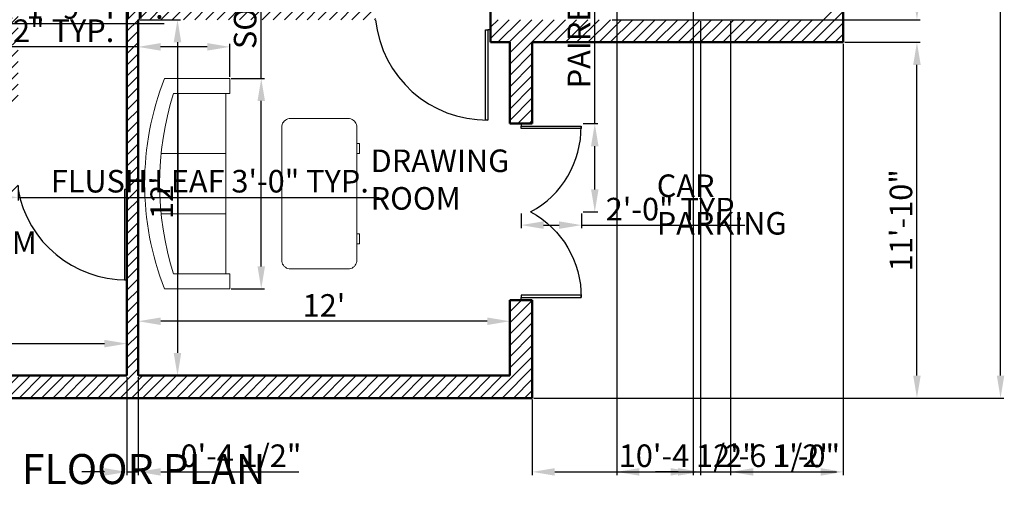
# Model space of a CAD drawing. Units: inches. Extents: x 5928 to 6612, y 5674 to 6320.
# Tile 2 of 5: x 6219 to 6612, y 5674 to 5862. Entities that reach past the tile are written whole.
import ezdxf

# ---------------------------------------------------------------- set-up
doc = ezdxf.new("R2010")
doc.units = ezdxf.units.IN
for name, color, linetype, lineweight in [('A-ANNO-DIMS', 2, 'Continuous', 18), ('A-ANNO-TEXT', 7, 'Continuous', 25), ('A-AREA-IDEN', 7, 'Continuous', 25), ('A-DOOR', 3, 'Continuous', 25), ('A-FURN', 8, 'Continuous', 18), ('A-WALL', 7, 'Continuous', 50), ('A-WALL-PATT', 252, 'Continuous', 13)]:
    doc.layers.add(name, color=color, linetype=linetype, lineweight=lineweight)
doc.styles.get("Standard").update_dxf_attribs({"font": 'arial.ttf'})
doc.dimstyles.new('ISO-25', dxfattribs={"dimtxt": 9, "dimasz": 9, "dimexe": 1.25, "dimexo": 0.625, "dimtad": 1, "dimdec": 1, "dimrnd": 9, "dimlunit": 3, "dimtxsty": 'Standard', "dimcen": 2.5, "dimadec": 0, "dimazin": 0, "dimtfac": 1, "dimtdec": 1, "dimtmove": 0, "dimatfit": 3, "dimfxl": 1, "dimarcsym": 0})

# ---------------------------------------------------------------- blocks, each defined once
blk = doc.blocks.new('Sofa - Roundback 7 ft.')
for p, q in [((-12.00002, -32.4421), (-12.00003, -6.5971)), ((11.99997, -32.4421), (11.99998, -6.5971)), ((-36.000027, -34), (-36.000027, -11.4696)), ((35.99998, -34), (35.99998, -11.4696)), ((-35.999844, -13.3819), (35.9998, -13.3819)), ((-36.000027, -32.4421), (35.99998, -32.4421))]:
    blk.add_line(p, q)
for points in [[(-36.000027, -34), (-42.000027, -34), (-42.000027, -8)], [(41.99998, -8), (41.99998, -34), (35.99998, -34)]]:
    blk.add_lwpolyline(points)
for centre, radius, start, end in [((0, -114.25), 114.25, 68.43141, 111.5686), ((-0.00001, -127.1968), 121.1968, 72.72033, 107.2797)]:
    blk.add_arc(centre, radius, start, end)
blk = doc.blocks.new('Desk - 30 x 60 in.')
for p, q in [((-26.999995, 0), (26.999995, 0)), ((-29.999995, -27), (-29.999995, -3)), ((29.999995, -3), (29.999995, -27)), ((26.999995, -30), (-26.999995, -30)), ((-20.000005, -30), (-20.000005, -31)), ((-20.000005, -31), (-16.000005, -31)), ((-16.000005, -31), (-16.000005, -30)), ((15.999995, -31), (15.999995, -30)), ((19.999995, -31), (15.999995, -31)), ((19.999995, -30), (19.999995, -31))]:
    blk.add_line(p, q)
for centre, start, end in [((-26.499995, -3.5), 98.1301, 171.8699), ((26.499995, -3.5), 8.130102, 81.8699), ((-26.499995, -26.5), 188.1301, 261.8699), ((26.499995, -26.5), 278.1301, 351.8699)]:
    blk.add_arc(centre, 3.535534, start, end)
blk = doc.blocks.new('*D20')
at = {"layer": 'A-ANNO-DIMS', "color": 0, "lineweight": -2, "transparency": 16777216}
for p, q in [((6117.76, 5720.89), (6117.76, 5734.25)), ((6261.76, 5720.89), (6261.76, 5734.25)), ((6126.76, 5733), (6252.76, 5733))]:
    blk.add_line(p, q, dxfattribs=at)
at = {"layer": 'A-ANNO-DIMS', "color": 0, "transparency": 16777216}
for points in [[(6126.76, 5734.5), (6126.76, 5731.5), (6117.76, 5733)], [(6252.76, 5734.5), (6252.76, 5731.5), (6261.76, 5733)]]:
    blk.add_solid(points, dxfattribs=at)
at = {"layer": 'Defpoints', "color": 0, "transparency": 16777216}
for p in [(6261.76, 5733), (6117.76, 5720.26), (6261.76, 5720.26)]:
    blk.add_point(p, dxfattribs=at)
at = {"layer": 'A-ANNO-DIMS', "color": 0, "transparency": 16777216, "insert": (6189.76, 5738.14), "char_height": 9, "attachment_point": 5}
blk.add_mtext("12'", dxfattribs=at)
blk = doc.blocks.new('*D21')
at = {"layer": 'A-ANNO-DIMS', "color": 0, "lineweight": -2, "transparency": 16777216}
for p, q in [((6266.88, 5862.26), (6283.21, 5862.26)), ((6281.96, 5853.26), (6281.96, 5729.26)), ((6266.88, 5720.26), (6283.21, 5720.26))]:
    blk.add_line(p, q, dxfattribs=at)
at = {"layer": 'A-ANNO-DIMS', "color": 0, "transparency": 16777216}
for points in [[(6280.46, 5853.26), (6283.46, 5853.26), (6281.96, 5862.26)], [(6280.46, 5729.26), (6283.46, 5729.26), (6281.96, 5720.26)]]:
    blk.add_solid(points, dxfattribs=at)
at = {"layer": 'Defpoints', "color": 0, "transparency": 16777216}
for p in [(6266.26, 5862.26), (6266.26, 5720.26), (6281.96, 5720.26)]:
    blk.add_point(p, dxfattribs=at)
at = {"layer": 'A-ANNO-DIMS', "color": 0, "transparency": 16777216, "insert": (6276.82, 5791.26), "char_height": 9, "attachment_point": 5, "rotation": 90}
blk.add_mtext("12'", dxfattribs=at)
blk = doc.blocks.new('*D22')
at = {"layer": 'A-ANNO-DIMS', "color": 0, "lineweight": -2, "transparency": 16777216}
for p, q in [((6266.26, 5720.89), (6266.26, 5743.18)), ((6405.76, 5741.93), (6275.26, 5741.93)), ((6414.76, 5720.89), (6414.76, 5743.18))]:
    blk.add_line(p, q, dxfattribs=at)
at = {"layer": 'A-ANNO-DIMS', "color": 0, "transparency": 16777216}
for points in [[(6275.26, 5743.43), (6275.26, 5740.43), (6266.26, 5741.93)], [(6405.76, 5743.43), (6405.76, 5740.43), (6414.76, 5741.93)]]:
    blk.add_solid(points, dxfattribs=at)
at = {"layer": 'Defpoints', "color": 0, "transparency": 16777216}
for p in [(6266.26, 5741.93), (6266.26, 5720.26), (6414.76, 5720.26)]:
    blk.add_point(p, dxfattribs=at)
at = {"layer": 'A-ANNO-DIMS', "color": 0, "transparency": 16777216, "insert": (6340.51, 5747.07), "char_height": 9, "attachment_point": 5}
blk.add_mtext("12'", dxfattribs=at)
blk = doc.blocks.new('*D37')
at = {"layer": 'A-ANNO-DIMS', "color": 0, "lineweight": -2, "transparency": 16777216}
for p, q in [((6497.65, 6228.26), (6612.14, 6228.26)), ((6610.89, 5720.26), (6610.89, 6219.26)), ((6424.38, 5711.26), (6612.14, 5711.26))]:
    blk.add_line(p, q, dxfattribs=at)
at = {"layer": 'A-ANNO-DIMS', "color": 0, "transparency": 16777216}
for points in [[(6609.39, 6219.26), (6612.39, 6219.26), (6610.89, 6228.26)], [(6609.39, 5720.26), (6612.39, 5720.26), (6610.89, 5711.26)]]:
    blk.add_solid(points, dxfattribs=at)
at = {"layer": 'Defpoints', "color": 0, "transparency": 16777216}
for p in [(6497.03, 6228.26), (6610.89, 6228.26), (6423.76, 5711.26)]:
    blk.add_point(p, dxfattribs=at)
at = {"layer": 'A-ANNO-DIMS', "color": 0, "transparency": 16777216, "insert": (6605.67, 5969.76), "char_height": 9, "attachment_point": 5, "rotation": 90}
blk.add_mtext('42\'-9"', dxfattribs=at)
blk = doc.blocks.new('DOOR-LEAF-36IN')
for p, q in [((0, 0), (0, 36)), ((0, 36), (1, 36)), ((1, 36), (1, 0)), ((-1, 0), (0, 0)), ((1, 0), (0, 0))]:
    blk.add_line(p, q)
blk = doc.blocks.new('DOOR-LEAF-FLUSH-36IN')
for p, q in [((0, 0), (-1, 0)), ((-1, 0), (-1, -36)), ((-1, -36), (0, -36))]:
    blk.add_line(p, q)
blk = doc.blocks.new('DOOR-PAIRED-LEAF-24IN')
for p, q in [((0, 0), (0, -1)), ((0, -1), (24, -1)), ((0, -2), (0, -1)), ((24, -2), (0, -2)), ((24, -1), (24, -2))]:
    blk.add_line(p, q)
blk.add_arc((-14.28, -1.5), 38.28, 298.2595, 0.7484)
blk = doc.blocks.new('*D49')
at = {"layer": 'A-ANNO-DIMS', "color": 0, "lineweight": -2, "transparency": 16777216}
for p, q in [((6191.35, 5865.09), (6191.35, 5859.51)), ((6212.35, 5865.09), (6212.35, 5859.51)), ((6200.35, 5860.76), (6203.35, 5860.76)), ((6212.35, 5860.76), (6276.61, 5860.76))]:
    blk.add_line(p, q, dxfattribs=at)
at = {"layer": 'A-ANNO-DIMS', "color": 0, "transparency": 16777216}
for points in [[(6200.35, 5862.26), (6200.35, 5859.26), (6191.35, 5860.76)], [(6203.35, 5862.26), (6203.35, 5859.26), (6212.35, 5860.76)]]:
    blk.add_solid(points, dxfattribs=at)
at = {"layer": 'Defpoints', "color": 0, "transparency": 16777216}
for p in [(6191.35, 5865.72), (6212.35, 5865.72), (6212.35, 5860.76)]:
    blk.add_point(p, dxfattribs=at)
at = {"layer": 'A-ANNO-DIMS', "color": 0, "transparency": 16777216, "insert": (6248.98, 5865.98), "char_height": 9, "attachment_point": 5}
blk.add_mtext('1\'-9" TYP.', dxfattribs=at)
blk = doc.blocks.new('*D54')
at = {"layer": 'A-ANNO-DIMS', "color": 0, "lineweight": -2, "transparency": 16777216}
for p, q in [((6315.43, 5838.83), (6315.43, 5941.63)), ((6303.46, 5838.83), (6316.68, 5838.83)), ((6315.43, 5763.83), (6315.43, 5829.83)), ((6303.46, 5754.83), (6316.68, 5754.83))]:
    blk.add_line(p, q, dxfattribs=at)
at = {"layer": 'A-ANNO-DIMS', "color": 0, "transparency": 16777216}
for points in [[(6313.93, 5829.83), (6316.93, 5829.83), (6315.43, 5838.83)], [(6313.93, 5763.83), (6316.93, 5763.83), (6315.43, 5754.83)]]:
    blk.add_solid(points, dxfattribs=at)
at = {"layer": 'Defpoints', "color": 0, "transparency": 16777216}
for p in [(6302.83, 5838.83), (6315.43, 5838.83), (6302.83, 5754.83)]:
    blk.add_point(p, dxfattribs=at)
at = {"layer": 'A-ANNO-DIMS', "color": 0, "transparency": 16777216, "insert": (6310.15, 5894.73), "char_height": 9, "attachment_point": 5, "rotation": 90}
blk.add_mtext('SOFA 7\'-0" TYP.', dxfattribs=at)
blk = doc.blocks.new('*D55')
at = {"layer": 'A-ANNO-DIMS', "color": 0, "lineweight": -2, "transparency": 16777216}
for p, q in [((6266.17, 5851.43), (6180.09, 5851.43)), ((6266.17, 5839.46), (6266.17, 5852.68)), ((6293.83, 5851.43), (6275.17, 5851.43)), ((6302.83, 5839.46), (6302.83, 5852.68))]:
    blk.add_line(p, q, dxfattribs=at)
at = {"layer": 'A-ANNO-DIMS', "color": 0, "transparency": 16777216}
for points in [[(6275.17, 5852.93), (6275.17, 5849.93), (6266.17, 5851.43)], [(6293.83, 5852.93), (6293.83, 5849.93), (6302.83, 5851.43)]]:
    blk.add_solid(points, dxfattribs=at)
at = {"layer": 'Defpoints', "color": 0, "transparency": 16777216}
for p in [(6266.17, 5851.43), (6266.17, 5838.83), (6302.83, 5838.83)]:
    blk.add_point(p, dxfattribs=at)
at = {"layer": 'A-ANNO-DIMS', "color": 0, "transparency": 16777216, "insert": (6218.63, 5856.72), "char_height": 9, "attachment_point": 5, "rotation": 360}
blk.add_mtext('3\'-0 1/2" TYP.', dxfattribs=at)
blk = doc.blocks.new('*D60')
at = {"layer": 'A-ANNO-DIMS', "color": 0, "lineweight": -2, "transparency": 16777216}
for p, q in [((6182.26, 5796.14), (6182.26, 5790.11)), ((6218.26, 5796.14), (6218.26, 5790.11)), ((6191.26, 5791.36), (6209.26, 5791.36)), ((6218.26, 5791.36), (6362.51, 5791.36))]:
    blk.add_line(p, q, dxfattribs=at)
at = {"layer": 'A-ANNO-DIMS', "color": 0, "transparency": 16777216}
for points in [[(6191.26, 5792.86), (6191.26, 5789.86), (6182.26, 5791.36)], [(6209.26, 5792.86), (6209.26, 5789.86), (6218.26, 5791.36)]]:
    blk.add_solid(points, dxfattribs=at)
at = {"layer": 'Defpoints', "color": 0, "transparency": 16777216}
for p in [(6182.26, 5796.76), (6218.26, 5796.76), (6218.26, 5791.36)]:
    blk.add_point(p, dxfattribs=at)
at = {"layer": 'A-ANNO-DIMS', "color": 0, "transparency": 16777216, "insert": (6294.88, 5796.65), "char_height": 9, "attachment_point": 5}
blk.add_mtext('FLUSH LEAF 3\'-0" TYP.', dxfattribs=at)
blk = doc.blocks.new('*D62')
at = {"layer": 'A-ANNO-DIMS', "color": 0, "lineweight": -2, "transparency": 16777216}
for p, q in [((6448.73, 5820.79), (6448.73, 5977.68)), ((6444.07, 5820.79), (6449.98, 5820.79)), ((6448.73, 5794.57), (6448.73, 5811.79)), ((6444.07, 5785.57), (6449.98, 5785.57))]:
    blk.add_line(p, q, dxfattribs=at)
at = {"layer": 'A-ANNO-DIMS', "color": 0, "transparency": 16777216}
for points in [[(6447.23, 5811.79), (6450.23, 5811.79), (6448.73, 5820.79)], [(6447.23, 5794.57), (6450.23, 5794.57), (6448.73, 5785.57)]]:
    blk.add_solid(points, dxfattribs=at)
at = {"layer": 'Defpoints', "color": 0, "transparency": 16777216}
for p in [(6443.45, 5820.79), (6448.73, 5820.79), (6443.45, 5785.57)]:
    blk.add_point(p, dxfattribs=at)
at = {"layer": 'A-ANNO-DIMS', "color": 0, "transparency": 16777216, "insert": (6443.58, 5903.73), "char_height": 9, "attachment_point": 5, "rotation": 90}
blk.add_mtext('PAIRED LEAF 2\'-11" TYP.', dxfattribs=at)
blk = doc.blocks.new('*D63')
at = {"layer": 'A-ANNO-DIMS', "color": 0, "lineweight": -2, "transparency": 16777216}
for p, q in [((6419.26, 5784.94), (6419.26, 5779.04)), ((6443.45, 5784.94), (6443.45, 5779.04)), ((6428.26, 5780.29), (6434.45, 5780.29)), ((6443.45, 5780.29), (6508.71, 5780.29))]:
    blk.add_line(p, q, dxfattribs=at)
at = {"layer": 'A-ANNO-DIMS', "color": 0, "transparency": 16777216}
for points in [[(6428.26, 5781.79), (6428.26, 5778.79), (6419.26, 5780.29)], [(6434.45, 5781.79), (6434.45, 5778.79), (6443.45, 5780.29)]]:
    blk.add_solid(points, dxfattribs=at)
at = {"layer": 'Defpoints', "color": 0, "transparency": 16777216}
for p in [(6419.26, 5785.57), (6443.45, 5785.57), (6443.45, 5780.29)]:
    blk.add_point(p, dxfattribs=at)
at = {"layer": 'A-ANNO-DIMS', "color": 0, "transparency": 16777216, "insert": (6480.58, 5785.51), "char_height": 9, "attachment_point": 5}
blk.add_mtext('2\'-0" TYP.', dxfattribs=at)
blk = doc.blocks.new('*D70')
at = {"layer": 'A-ANNO-DIMS', "color": 0, "lineweight": -2, "transparency": 16777216}
for p, q in [((6548.03, 5852.64), (6548.03, 5680.56)), ((6423.76, 5710.64), (6423.76, 5680.56)), ((6432.76, 5681.81), (6539.03, 5681.81))]:
    blk.add_line(p, q, dxfattribs=at)
at = {"layer": 'A-ANNO-DIMS', "color": 0, "transparency": 16777216}
for points in [[(6432.76, 5683.31), (6432.76, 5680.31), (6423.76, 5681.81)], [(6539.03, 5683.31), (6539.03, 5680.31), (6548.03, 5681.81)]]:
    blk.add_solid(points, dxfattribs=at)
at = {"layer": 'Defpoints', "color": 0, "transparency": 16777216}
for p in [(6548.03, 5853.26), (6423.76, 5711.26), (6548.03, 5681.81)]:
    blk.add_point(p, dxfattribs=at)
at = {"layer": 'A-ANNO-DIMS', "color": 0, "transparency": 16777216, "insert": (6485.89, 5687.09), "char_height": 9, "attachment_point": 5}
blk.add_mtext('10\'-4 1/2"', dxfattribs=at)
blk = doc.blocks.new('*D71')
at = {"layer": 'A-ANNO-DIMS', "color": 0, "lineweight": -2, "transparency": 16777216}
for p, q in [((6548.65, 5853.26), (6578.73, 5853.26)), ((6577.48, 5720.26), (6577.48, 5844.26)), ((6424.38, 5711.26), (6578.73, 5711.26))]:
    blk.add_line(p, q, dxfattribs=at)
at = {"layer": 'A-ANNO-DIMS', "color": 0, "transparency": 16777216}
for points in [[(6575.98, 5844.26), (6578.98, 5844.26), (6577.48, 5853.26)], [(6575.98, 5720.26), (6578.98, 5720.26), (6577.48, 5711.26)]]:
    blk.add_solid(points, dxfattribs=at)
at = {"layer": 'Defpoints', "color": 0, "transparency": 16777216}
for p in [(6548.03, 5853.26), (6577.48, 5853.26), (6423.76, 5711.26)]:
    blk.add_point(p, dxfattribs=at)
at = {"layer": 'A-ANNO-DIMS', "color": 0, "transparency": 16777216, "insert": (6572.26, 5782.26), "char_height": 9, "attachment_point": 5, "rotation": 90}
blk.add_mtext('11\'-10"', dxfattribs=at)
blk = doc.blocks.new('*D76')
at = {"layer": 'A-ANNO-DIMS', "color": 0, "lineweight": -2, "transparency": 16777216}
for p, q in [((6261.76, 5719.64), (6261.76, 5680.56)), ((6266.26, 5719.64), (6266.26, 5680.56)), ((6252.76, 5681.81), (6243.76, 5681.81)), ((6261.76, 5681.81), (6266.26, 5681.81)), ((6275.26, 5681.81), (6330.41, 5681.81))]:
    blk.add_line(p, q, dxfattribs=at)
at = {"layer": 'A-ANNO-DIMS', "color": 0, "transparency": 16777216}
for points in [[(6252.76, 5683.31), (6252.76, 5680.31), (6261.76, 5681.81)], [(6275.26, 5683.31), (6275.26, 5680.31), (6266.26, 5681.81)]]:
    blk.add_solid(points, dxfattribs=at)
at = {"layer": 'Defpoints', "color": 0, "transparency": 16777216}
for p in [(6261.76, 5720.26), (6266.26, 5720.26), (6266.26, 5681.81)]:
    blk.add_point(p, dxfattribs=at)
at = {"layer": 'A-ANNO-DIMS', "color": 0, "transparency": 16777216, "insert": (6307.33, 5687.09), "char_height": 9, "attachment_point": 5}
blk.add_mtext('0\'-4 1/2"', dxfattribs=at)
blk = doc.blocks.new('*D77')
at = {"layer": 'A-ANNO-DIMS', "color": 0, "lineweight": -2, "transparency": 16777216}
for p, q in [((6457.49, 5974.14), (6457.49, 5680.56)), ((6488.03, 5974.14), (6488.03, 5680.56)), ((6466.49, 5681.81), (6479.03, 5681.81)), ((6488.03, 5681.81), (6543.33, 5681.81))]:
    blk.add_line(p, q, dxfattribs=at)
at = {"layer": 'A-ANNO-DIMS', "color": 0, "transparency": 16777216}
for points in [[(6466.49, 5683.31), (6466.49, 5680.31), (6457.49, 5681.81)], [(6479.03, 5683.31), (6479.03, 5680.31), (6488.03, 5681.81)]]:
    blk.add_solid(points, dxfattribs=at)
at = {"layer": 'Defpoints', "color": 0, "transparency": 16777216}
for p in [(6457.49, 5974.76), (6488.03, 5974.76), (6488.03, 5681.81)]:
    blk.add_point(p, dxfattribs=at)
at = {"layer": 'A-ANNO-DIMS', "color": 0, "transparency": 16777216, "insert": (6520.18, 5687.09), "char_height": 9, "attachment_point": 5}
blk.add_mtext('2\'-6 1/2"', dxfattribs=at)
blk = doc.blocks.new('*D78')
at = {"layer": 'A-ANNO-DIMS', "color": 0, "lineweight": -2, "transparency": 16777216}
for p, q in [((6455.65, 5916.26), (6578.73, 5916.26)), ((6577.48, 5871.26), (6577.48, 5907.26)), ((6455.65, 5862.26), (6578.73, 5862.26))]:
    blk.add_line(p, q, dxfattribs=at)
at = {"layer": 'A-ANNO-DIMS', "color": 0, "transparency": 16777216}
for points in [[(6575.98, 5907.26), (6578.98, 5907.26), (6577.48, 5916.26)], [(6575.98, 5871.26), (6578.98, 5871.26), (6577.48, 5862.26)]]:
    blk.add_solid(points, dxfattribs=at)
at = {"layer": 'Defpoints', "color": 0, "transparency": 16777216}
for p in [(6455.03, 5916.26), (6577.48, 5916.26), (6455.03, 5862.26)]:
    blk.add_point(p, dxfattribs=at)
at = {"layer": 'A-ANNO-DIMS', "color": 0, "transparency": 16777216, "insert": (6572.26, 5889.26), "char_height": 9, "attachment_point": 5, "rotation": 90}
blk.add_mtext('4\'-6"', dxfattribs=at)
blk = doc.blocks.new('*D79')
at = {"layer": 'A-ANNO-DIMS', "color": 0, "lineweight": -2, "transparency": 16777216}
for p, q in [((6491.03, 5861.64), (6491.03, 5680.56)), ((6503.03, 5861.64), (6503.03, 5680.56)), ((6482.03, 5681.81), (6473.03, 5681.81)), ((6491.03, 5681.81), (6503.03, 5681.81)), ((6512.03, 5681.81), (6545.35, 5681.81))]:
    blk.add_line(p, q, dxfattribs=at)
at = {"layer": 'A-ANNO-DIMS', "color": 0, "transparency": 16777216}
for points in [[(6482.03, 5683.31), (6482.03, 5680.31), (6491.03, 5681.81)], [(6512.03, 5683.31), (6512.03, 5680.31), (6503.03, 5681.81)]]:
    blk.add_solid(points, dxfattribs=at)
at = {"layer": 'Defpoints', "color": 0, "transparency": 16777216}
for p in [(6491.03, 5862.26), (6503.03, 5862.26), (6503.03, 5681.81)]:
    blk.add_point(p, dxfattribs=at)
at = {"layer": 'A-ANNO-DIMS', "color": 0, "transparency": 16777216, "insert": (6533.19, 5687.03), "char_height": 9, "attachment_point": 5}
blk.add_mtext('1\'-0"', dxfattribs=at)

msp = doc.modelspace()

# ---------------------------------------------------------------- hatches: boundary and pattern name
at = {"layer": 'A-WALL-PATT'}
h = msp.add_hatch(dxfattribs=at)
h.set_pattern_fill('ANSI31', color=256)
h.paths.add_polyline_path([(6071.03, 6165.76), (6215.03, 6165.76), (6215.03, 5969.77), (6215.03, 5950.32), (6219.53, 5950.32), (6219.53, 6142.76), (6239.11, 6142.76), (6239.11, 6151.76), (6224.03, 6151.76), (6224.03, 6174.76), (6062.03, 6174.76), (6062.03, 5969.76), (6062.03, 5894.26), (6108.76, 5894.26), (6108.76, 5711.26), (6423.76, 5711.26), (6423.76, 5750.35), (6414.76, 5750.35), (6414.76, 5720.26), (6266.26, 5720.26), (6266.26, 5862.26), (6361.1, 5862.26), (6361.1, 5866.76), (6261.76, 5866.76), (6261.76, 5720.26), (6117.76, 5720.26), (6117.76, 5792.26), (6218.26, 5792.26), (6218.26, 5796.76), (6117.76, 5796.76), (6117.76, 5898.76), (6213.76, 5898.76), (6213.76, 5828.21, -0.018207), (6216.01, 5828.09), (6218.26, 5828.09), (6218.26, 5903.26), (6117.76, 5903.26), (6071.03, 5903.26), (6071.03, 5969.77), (6071.03, 6041.26), (6117.76, 6041.26), (6172.44, 6041.26), (6172.44, 6045.76), (6117.76, 6045.76), (6071.03, 6045.76)])
h.paths.add_polyline_path([(6368.03, 6219.26), (6488.03, 6219.26), (6488.03, 6147.26), (6403.79, 6147.26), (6403.79, 6142.76), (6488.03, 6142.76), (6488.03, 5974.76), (6363.53, 5974.76), (6363.53, 5970.11), (6497.03, 5970.26), (6497.03, 6142.76), (6497.03, 6228.26), (6359.03, 6228.26), (6359.03, 6151.76), (6344.11, 6151.76), (6344.11, 6142.76), (6363.53, 6142.76), (6363.53, 6013.35), (6368.03, 6013.35), (6368.03, 6142.76)])
h.paths.add_polyline_path([(6344.11, 6196.21, 0.265753), (6295.16, 6228.26), (6288.06, 6228.26, 0.265753), (6239.11, 6196.21), (6239.11, 6142.76), (6243.61, 6142.76), (6243.61, 6196.76), (6243.45, 6196.76, -0.514089), (6339.79, 6196.74), (6339.61, 6196.76), (6339.61, 6142.76), (6344.11, 6142.76)])
h.paths.add_polyline_path([(6339.61, 6147.26), (6327.61, 6147.26), (6327.61, 6142.76), (6339.61, 6142.76)], flags=17)
h.paths.add_polyline_path([(6255.61, 6147.26), (6243.61, 6147.26), (6243.61, 6142.76), (6255.61, 6142.76)], flags=17)
h.paths.add_polyline_path([(6548.03, 5974.76), (6539.03, 5974.76), (6539.03, 5862.26), (6407.03, 5862.26), (6407.03, 5853.26), (6414.76, 5853.26), (6414.76, 5820.79), (6423.76, 5820.79), (6423.76, 5853.26), (6548.03, 5853.26)])

# ---------------------------------------------------------------- linework, layer by layer
at = {"layer": 'A-DOOR'}
for centre, radius, start, end in [((6405.53, 5866.89), 44.67, 185.9456, 270.6414), ((6261.26, 5802.19), 43.68, 190.1228, 270.6559)]:
    msp.add_arc(centre, radius, start, end, dxfattribs=at)
at = {"layer": 'A-WALL'}
for p, q in [((6548.03, 5853.26), (6548.03, 5974.76)), ((6407.03, 5853.26), (6407.03, 5916.26)), ((6261.76, 5866.76), (6261.76, 5720.26)), ((6266.26, 5862.26), (6266.26, 5720.26)), ((6414.76, 5853.26), (6407.03, 5853.26)), ((6414.76, 5853.26), (6414.76, 5820.79)), ((6548.03, 5853.26), (6423.76, 5853.26)), ((6423.76, 5853.26), (6423.76, 5820.79)), ((6423.76, 5820.79), (6414.76, 5820.79)), ((6423.76, 5750.35), (6414.76, 5750.35)), ((6414.76, 5750.35), (6414.76, 5720.26)), ((6423.76, 5750.35), (6423.76, 5711.26)), ((6117.76, 5720.26), (6261.76, 5720.26)), ((6266.26, 5720.26), (6414.76, 5720.26)), ((6108.76, 5711.26), (6423.76, 5711.26))]:
    msp.add_line(p, q, dxfattribs=at)

# ---------------------------------------------------------------- block references
at = {"layer": 'A-DOOR', "rotation": 180}
msp.add_blockref('DOOR-LEAF-36IN', (6406.03, 5858.23), dxfattribs=at)
at = {"layer": 'A-DOOR'}
for name, p in [('DOOR-PAIRED-LEAF-24IN', (6419.26, 5820.79)), ('DOOR-LEAF-FLUSH-36IN', (6261.76, 5794.51))]:
    msp.add_blockref(name, p, dxfattribs=at)
at = {"layer": 'A-DOOR', "extrusion": (0, 0, -1), "zscale": -1, "rotation": 180}
msp.add_blockref('DOOR-PAIRED-LEAF-24IN', (-6419.26, 5750.35), dxfattribs=at)
at = {"layer": 'A-FURN'}
for name, p, rotation in [('Sofa - Roundback 7 ft.', (6268.83, 5796.83), 89.99997444959332), ('Desk - 30 x 60 in.', (6323.64, 5792.82), 90)]:
    msp.add_blockref(name, p, dxfattribs=dict(at, rotation=rotation))

# ---------------------------------------------------------------- texts
at = {"layer": 'A-ANNO-TEXT', "insert": (6147.39, 5688.94), "char_height": 12, "attachment_point": 1}
msp.add_mtext_dynamic_manual_height_columns('GROUND FLOOR PLAN', width=356.796, gutter_width=12.5, heights=[0], dxfattribs=at)
at = {"layer": 'A-AREA-IDEN', "char_height": 9, "attachment_point": 1}
for s, width, heights, insert in [('DRAWING\\PROOM', 104.7589, [0], (6359.14, 5810.47)), ('CAR PARKING', 64.9053, [0], (6473.49, 5800.51)), ('BED ROOM', 64.9053, [24.31], (6163.21, 5777.76))]:
    msp.add_mtext_dynamic_manual_height_columns(s, width=width, gutter_width=12.5, heights=heights, dxfattribs=dict(at, insert=insert))

# ---------------------------------------------------------------- dimensions: what is measured, and where the dimension line sits
at = {"layer": 'A-ANNO-DIMS'}
for base, p1, p2, override, picture, middle in [((6610.89, 6228.26), (6423.76, 5711.26), (6497.03, 6228.26), {"dimclrd": 0, "dimclre": 0, "dimclrt": 0}, '*D37', (6605.67, 5969.76)), ((6577.48, 5916.26), (6455.03, 5862.26), (6455.03, 5916.26), {"dimdec": 1, "dimlfac": 1, "dimrnd": 0, "dimzin": 1, "dimdsep": 46, "dimlunit": 4, "dimfrac": 2}, '*D78', (6572.26, 5889.26)), ((6281.96, 5720.26), (6266.26, 5862.26), (6266.26, 5720.26), {"dimclrd": 0, "dimclre": 0, "dimclrt": 0}, '*D21', (6276.82, 5791.26)), ((6577.48, 5853.26), (6423.76, 5711.26), (6548.03, 5853.26), {"dimdec": 1, "dimlfac": 1, "dimrnd": 0, "dimzin": 1, "dimdsep": 46, "dimlunit": 4, "dimfrac": 2}, '*D71', (6572.26, 5782.26))]:
    dim = msp.add_linear_dim(base=base, p1=p1, p2=p2, angle=90, dimstyle='ISO-25', override=override, dxfattribs=at)
    dim.commit()
    dim.dimension.update_dxf_attribs({"geometry": picture, "text_midpoint": middle})
for base, p1, p2, angle, text, picture, middle in [((6448.73, 5820.79), (6443.45, 5785.57), (6443.45, 5820.79), 90, 'PAIRED LEAF <> TYP.', '*D62', (6443.58, 5903.73)), ((6315.43, 5838.83), (6302.83, 5754.83), (6302.83, 5838.83), 90, 'SOFA <> TYP.', '*D54', (6310.15, 5894.73)), ((6266.17, 5851.43), (6302.83, 5838.83), (6266.17, 5838.83), 180, '<> TYP.', '*D55', (6218.63, 5856.72)), ((6218.26, 5791.36), (6182.26, 5796.76), (6218.26, 5796.76), 0, 'FLUSH LEAF <> TYP.', '*D60', (6294.88, 5796.65))]:
    dim = msp.add_linear_dim(base=base, p1=p1, p2=p2, angle=angle, text=text, dimstyle='ISO-25', override={"dimdec": 1, "dimlfac": 1, "dimrnd": 0, "dimzin": 1, "dimdsep": 46, "dimlunit": 4, "dimfrac": 2}, dxfattribs=at)
    dim.commit()
    dim.dimension.update_dxf_attribs({"geometry": picture, "text_midpoint": middle})
for base, p1, p2, override, picture, middle in [((6488.03, 5681.81), (6457.49, 5974.76), (6488.03, 5974.76), {"dimdec": 1, "dimlfac": 1, "dimrnd": 0, "dimzin": 1, "dimdsep": 46, "dimlunit": 4, "dimfrac": 2}, '*D77', (6520.18, 5687.09)), ((6503.03, 5681.81), (6491.03, 5862.26), (6503.03, 5862.26), {"dimdec": 1, "dimlfac": 1, "dimrnd": 0, "dimzin": 1, "dimdsep": 46, "dimlunit": 4, "dimfrac": 2}, '*D79', (6533.19, 5687.03)), ((6548.03, 5681.81), (6423.76, 5711.26), (6548.03, 5853.26), {"dimdec": 1, "dimlfac": 1, "dimrnd": 0, "dimzin": 1, "dimdsep": 46, "dimlunit": 4, "dimfrac": 2}, '*D70', (6485.89, 5687.09)), ((6266.26, 5741.93), (6414.76, 5720.26), (6266.26, 5720.26), {"dimclrd": 0, "dimclre": 0, "dimclrt": 0}, '*D22', (6340.51, 5747.07)), ((6261.76, 5733), (6117.76, 5720.26), (6261.76, 5720.26), {"dimclrd": 0, "dimclre": 0, "dimclrt": 0}, '*D20', (6189.76, 5738.14)), ((6266.26, 5681.81), (6261.76, 5720.26), (6266.26, 5720.26), {"dimdec": 1, "dimlfac": 1, "dimrnd": 0, "dimzin": 1, "dimdsep": 46, "dimlunit": 4, "dimfrac": 2}, '*D76', (6307.33, 5687.09))]:
    dim = msp.add_linear_dim(base=base, p1=p1, p2=p2, dimstyle='ISO-25', override=override, dxfattribs=at)
    dim.commit()
    dim.dimension.update_dxf_attribs({"geometry": picture, "text_midpoint": middle})
for base, p1, p2, picture, middle in [((6212.35, 5860.76), (6191.35, 5865.72), (6212.35, 5865.72), '*D49', (6248.98, 5865.98)), ((6443.45, 5780.29), (6419.26, 5785.57), (6443.45, 5785.57), '*D63', (6480.58, 5785.51))]:
    dim = msp.add_linear_dim(base=base, p1=p1, p2=p2, text='<> TYP.', dimstyle='ISO-25', override={"dimdec": 1, "dimlfac": 1, "dimrnd": 0, "dimzin": 1, "dimdsep": 46, "dimlunit": 4, "dimfrac": 2}, dxfattribs=at)
    dim.commit()
    dim.dimension.update_dxf_attribs({"geometry": picture, "text_midpoint": middle})

doc.saveas('drawing.dxf')
